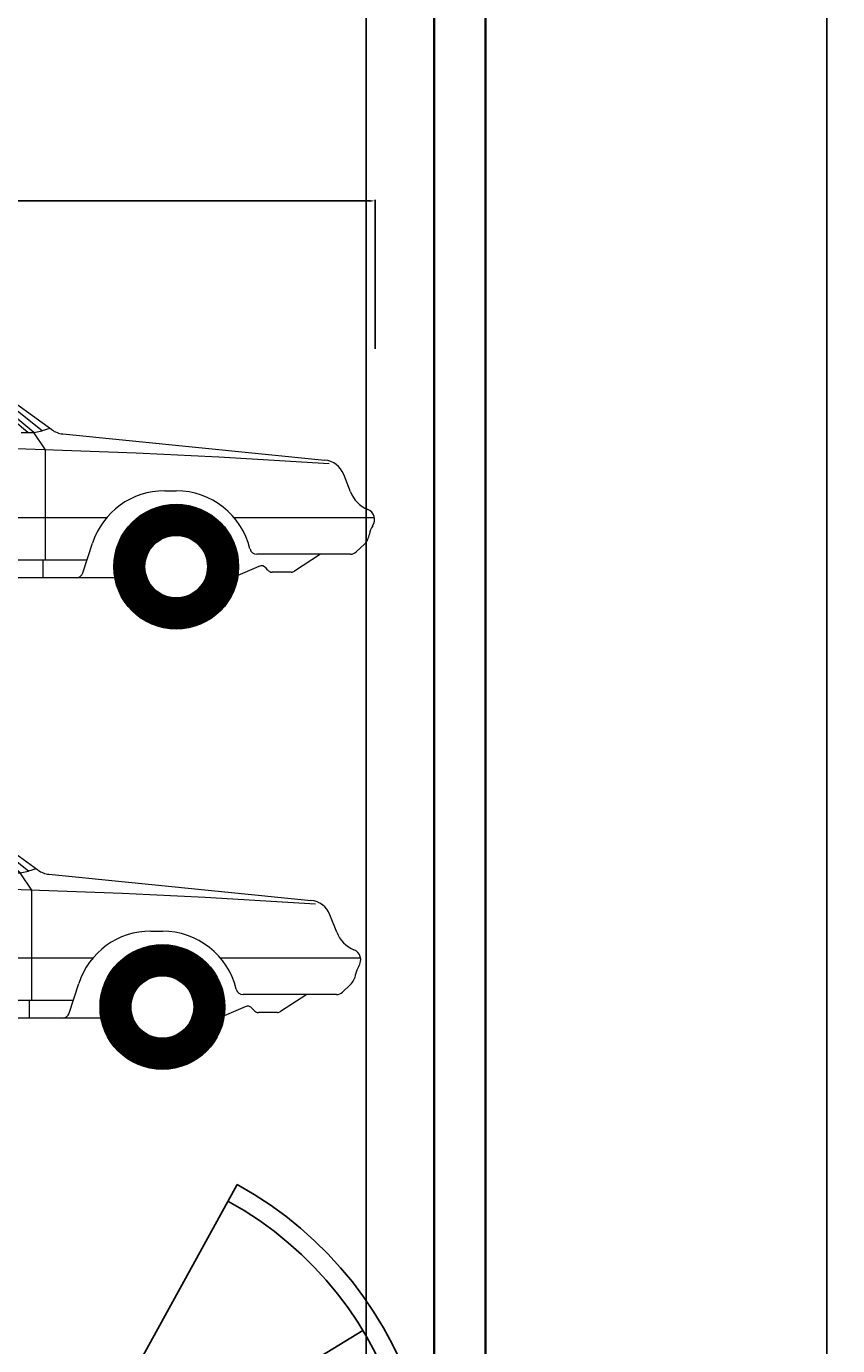
# Model space of a CAD drawing. Units: inches. Extents: x 371 to 1095, y -45 to 1219.
# Tile 7 of 18: x 952 to 1095, y 188 to 421. Entities that reach past the tile are written whole.
import ezdxf

# ---------------------------------------------------------------- set-up
doc = ezdxf.new("R2010")
doc.units = ezdxf.units.IN
doc.header["$MEASUREMENT"] = 0
for name, color, linetype, lineweight in [('A-ANNO-DIMS', 2, 'Continuous', 18), ('A-FLOR-STRS', 7, 'Continuous', 25), ('A-WALL', 40, 'Continuous', 35), ('C-SITE-VEHC', 8, 'Continuous', 18), ('C-SITE-WALL', 40, 'Continuous', 35)]:
    doc.layers.add(name, color=color, linetype=linetype, lineweight=lineweight)
doc.styles.get("Standard").update_dxf_attribs({"font": 'arial.ttf'})
doc.dimstyles.get("Standard").update_dxf_attribs({"dimtxt": 1, "dimasz": 1, "dimexe": 0.18, "dimexo": 0.0625, "dimgap": 0.09, "dimtad": 0, "dimtih": 1, "dimtoh": 1, "dimdec": 0, "dimzin": 0, "dimdsep": 46, "dimlunit": 3, "dimtxsty": 'Standard', "dimcen": 0.09, "dimadec": 0, "dimazin": 0, "dimtfac": 1, "dimtdec": 0, "dimtofl": 0, "dimtmove": 0, "dimatfit": 3, "dimfxl": 1, "dimtolj": 1, "dimtzin": 0, "dimarcsym": 0})

# ---------------------------------------------------------------- blocks, each defined once
blk = doc.blocks.new('Staircase - Spiral')
for p, q in [((4.5, 0), (30, 0)), ((3.8999, -2.2518), (24.6817, -14.2502))]:
    blk.add_line(p, q)
for radius in [30, 28.5]:
    blk.add_arc((0, 0), radius, 90, 0)
blk = doc.blocks.new('Car - sedan  side')
for p, q in [((-61.08, 34.66), (-76.26, 47.3)), ((-60.02, 34.65), (-76.07, 48.02)), ((-56.87, 35.13), (-75.48, 48.59)), ((-58.54, 34.93), (-74.99, 48.02)), ((-60.02, 34.65), (-58.54, 34.93)), ((-57.21, 35.38), (-58.54, 34.93)), ((-62.28, 34.67), (-60.02, 34.65)), ((-57.97, 31.61), (-60.02, 34.65)), ((-54.93, 34.4), (-8.75, 29.8)), ((-57.97, 19.62), (-57.97, 31.61)), ((-4.21, 24.18), (-5.42, 27.27)), ((-36.97, 24.38), (-34.94, 24.38)), ((-47.2, 19.62), (-125.23, 19.62)), ((-57.97, 12.14), (-57.97, 19.62)), ((0, 19.62), (-24.7, 19.62)), ((-51.4, 9.89), (-49.69, 15.14)), ((-3.22, 13.59), (-1.77, 14.97)), ((-50.67, 12.14), (-123.32, 12.14)), ((-58.39, 9.03), (-58.39, 12.14)), ((-4.23, 13.19), (-20.72, 13.19)), ((-9.5, 13.19), (-14.1, 10.2)), ((-20.36, 11.06), (-24.06, 9.44)), ((-18.83, 10.42), (-19.11, 10.76)), ((-14.68, 10.03), (-18.01, 10.03)), ((-45.76, 9.03), (-120.62, 9.03))]:
    blk.add_line(p, q)
at = {"const_width": 5.49}
blk.add_lwpolyline([(-26.69, 11, -1), (-43.19, 11, -1)], format="xyb", close=True, dxfattribs=at)
for radius in [11, 5.51]:
    blk.add_circle((-34.94, 11), radius)
for centre, radius, start, end in [((-54.54, 38.35), 3.97, 234.135, 264.3123), ((-118.51, -1702.12), 1734.79, 86.34698, 91.49105), ((-9.15, 25.82), 4, 21.3107, 84.3123), ((-36.97, 11), 13.38, 90, 161.9732), ((-34.94, 11), 13.38, 13.5864, 90), ((0.9, 26.18), 5.49, 201.3107, 247.7048), ((-1.92, 19.3), 1.94, 325.3744, 67.7048), ((-3.82, 17.12), 2.96, 313.7173, 352.3839), ((2.46, 16.28), 3.37, 145.3744, 172.3839), ((-20.72, 14.43), 1.24, 193.5864, 270), ((-4.23, 14.65), 1.46, 270, 313.7173), ((-52.58, 10.27), 1.24, 270, 341.9732), ((-19.93, 10.09), 1.06, 39.301, 113.7159), ((-18.01, 11.09), 1.06, 219.301, 270), ((-14.68, 11.09), 1.06, 270, 303.047)]:
    blk.add_arc(centre, radius, start, end)
blk = doc.blocks.new('*D38')
at = {"layer": 'A-ANNO-DIMS', "color": 0, "lineweight": -2, "transparency": 16777216}
for p, q in [((839.26, 363.91), (839.26, 390.15)), ((840.26, 389.97), (920.19, 389.97)), ((1012.37, 389.97), (932.44, 389.97)), ((1013.37, 363.91), (1013.37, 390.15))]:
    blk.add_line(p, q, dxfattribs=at)
at = {"layer": 'A-ANNO-DIMS', "color": 0, "transparency": 16777216}
for points in [[(840.26, 390.13), (840.26, 389.8), (839.26, 389.97)], [(1012.37, 390.13), (1012.37, 389.8), (1013.37, 389.97)]]:
    blk.add_solid(points, dxfattribs=at)
at = {"layer": 'Defpoints', "color": 0, "transparency": 16777216}
for p in [(1013.37, 389.97), (839.26, 363.85), (1013.37, 363.85)]:
    blk.add_point(p, dxfattribs=at)
at = {"layer": 'A-ANNO-DIMS', "color": 0, "transparency": 16777216, "insert": (926.31, 389.97), "char_height": 1, "attachment_point": 5}
blk.add_mtext('\\A1;SEDAN 14\'-6" TYP.', dxfattribs=at)
blk = doc.blocks.new('*D51')
at = {"layer": 'A-ANNO-DIMS', "color": 0, "lineweight": -2, "transparency": 16777216}
for p, q in [((1032.87, 982.03), (1093.19, 982.03)), ((1093.01, 981.03), (1093.01, 532.63)), ((1093.01, 83.03), (1093.01, 531.42)), ((1032.87, 82.03), (1093.19, 82.03))]:
    blk.add_line(p, q, dxfattribs=at)
at = {"layer": 'A-ANNO-DIMS', "color": 0, "transparency": 16777216}
for points in [[(1092.84, 981.03), (1093.17, 981.03), (1093.01, 982.03)], [(1092.84, 83.03), (1093.17, 83.03), (1093.01, 82.03)]]:
    blk.add_solid(points, dxfattribs=at)
at = {"layer": 'Defpoints', "color": 0, "transparency": 16777216}
for p in [(1032.81, 982.03), (1093.01, 982.03), (1032.81, 82.03)]:
    blk.add_point(p, dxfattribs=at)
at = {"layer": 'A-ANNO-DIMS', "color": 0, "transparency": 16777216, "insert": (1093.01, 532.03), "char_height": 1, "attachment_point": 5}
blk.add_mtext('\\A1;75\'-0"', dxfattribs=at)
blk = doc.blocks.new('*D62')
at = {"layer": 'A-ANNO-DIMS', "color": 0, "lineweight": -2, "transparency": 16777216}
for p, q in [((1023.81, 450.96), (1023.81, -43.83)), ((1011.81, 441.96), (1011.81, -43.83)), ((1012.81, -43.65), (1016.44, -43.65)), ((1022.81, -43.65), (1019.18, -43.65))]:
    blk.add_line(p, q, dxfattribs=at)
at = {"layer": 'A-ANNO-DIMS', "color": 0, "transparency": 16777216}
for points in [[(1012.81, -43.48), (1012.81, -43.82), (1011.81, -43.65)], [(1022.81, -43.48), (1022.81, -43.82), (1023.81, -43.65)]]:
    blk.add_solid(points, dxfattribs=at)
at = {"layer": 'Defpoints', "color": 0, "transparency": 16777216}
for p in [(1023.81, 451.03), (1011.81, 442.03), (1023.81, -43.65)]:
    blk.add_point(p, dxfattribs=at)
at = {"layer": 'A-ANNO-DIMS', "color": 0, "transparency": 16777216, "insert": (1017.81, -43.65), "char_height": 1, "attachment_point": 5}
blk.add_mtext('\\A1;1\'-0"', dxfattribs=at)

msp = doc.modelspace()

# ---------------------------------------------------------------- linework, layer by layer
at = {"layer": 'A-WALL'}
msp.add_line((1032.81, 82.03), (1032.81, 982.03), dxfattribs=at)
at = {"layer": 'C-SITE-WALL'}
msp.add_line((1023.81, 91.03), (1023.81, 442.03), dxfattribs=at)

# ---------------------------------------------------------------- block references
at = {"layer": 'A-FLOR-STRS', "xscale": 2.233824712970382, "yscale": 2.233824712970382, "zscale": 2.233824712970382, "rotation": 61.2124779579666}
msp.add_blockref('Staircase - Spiral', (956.78, 157.87), dxfattribs=at)
at = {"layer": 'C-SITE-VEHC'}
for p in [(1013.26, 314.5), (1010.83, 236.89)]:
    msp.add_blockref('Car - sedan  side', p, dxfattribs=at)

# ---------------------------------------------------------------- dimensions: what is measured, and where the dimension line sits
at = {"layer": 'A-ANNO-DIMS'}
dim = msp.add_linear_dim(base=(1093.01, 982.03), p1=(1032.81, 82.03), p2=(1032.81, 982.03), angle=90, dimstyle='Standard', override={"dimdec": 1, "dimlfac": 1, "dimrnd": 0, "dimzin": 1, "dimdsep": 46, "dimlunit": 4, "dimfrac": 2}, dxfattribs=at)
dim.commit()
dim.dimension.update_dxf_attribs({"geometry": '*D51', "text_midpoint": (1093.01, 532.03)})
dim = msp.add_linear_dim(base=(1023.81, -43.65), p1=(1011.81, 442.03), p2=(1023.81, 451.03), dimstyle='Standard', override={"dimdec": 1, "dimlfac": 1, "dimrnd": 0, "dimzin": 1, "dimdsep": 46, "dimlunit": 4, "dimfrac": 2}, dxfattribs=at)
dim.commit()
dim.dimension.update_dxf_attribs({"geometry": '*D62', "text_midpoint": (1017.81, -43.65)})
dim = msp.add_linear_dim(base=(1013.37, 389.97), p1=(839.26, 363.85), p2=(1013.37, 363.85), text='SEDAN <> TYP.', dimstyle='Standard', override={"dimdec": 1, "dimlfac": 1, "dimrnd": 0, "dimzin": 1, "dimdsep": 46, "dimlunit": 4, "dimfrac": 2}, dxfattribs=at)
dim.commit()
dim.dimension.update_dxf_attribs({"geometry": '*D38', "text_midpoint": (926.31, 389.97)})

doc.saveas('drawing.dxf')
